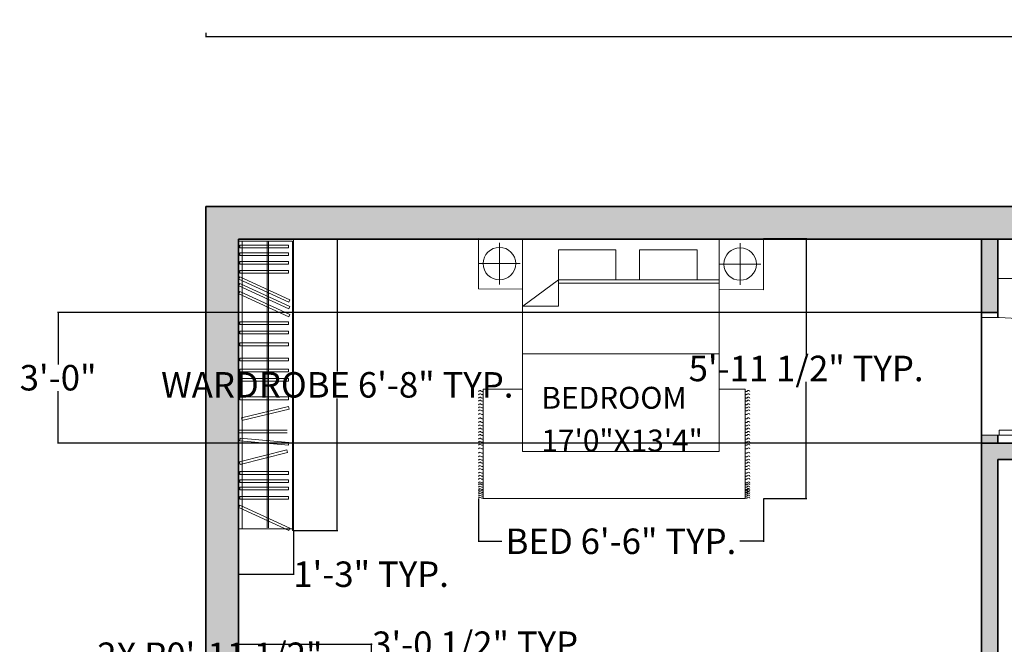
# Model space of a CAD drawing. Units: inches. Extents: x 1319 to 2030, y 219 to 1069.
# Tile 25 of 28: x 1319 to 1589, y 835 to 1007. Entities that reach past the tile are written whole.
import ezdxf

# ---------------------------------------------------------------- set-up
doc = ezdxf.new("R2010")
doc.units = ezdxf.units.IN
doc.header["$MEASUREMENT"] = 0
doc.layers.get('0').update_dxf_attribs({"color": 12})
for name, color, linetype, lineweight in [('A-ANNO-DIMS', 2, 'Continuous', 18), ('A-AREA-IDEN', 250, 'Continuous', 18), ('A-WALL-PATT', 252, 'Continuous', 13), ('C-PROP', 7, 'Continuous', 35), ('closet', 252, 'Continuous', 18), ('doors', 252, 'Continuous', 18), ('furniture', 250, 'Continuous', 18), ('walls', 250, 'Continuous', 35)]:
    doc.layers.add(name, color=color, linetype=linetype, lineweight=lineweight)
doc.styles.get("Standard").update_dxf_attribs({"font": 'arial.ttf'})
doc.dimstyles.get("Standard").update_dxf_attribs({"dimtxt": 7, "dimasz": 0.18, "dimexe": 0.18, "dimexo": 0.0625, "dimgap": 0.09, "dimtad": 0, "dimtih": 1, "dimtoh": 1, "dimzin": 0, "dimdsep": 46, "dimlunit": 3, "dimtxsty": 'Standard', "dimcen": 0.09, "dimadec": 0, "dimazin": 0, "dimtfac": 1, "dimtofl": 0, "dimtmove": 0, "dimatfit": 3, "dimfxl": 1, "dimtolj": 1, "dimtzin": 0, "dimarcsym": 0})

# ---------------------------------------------------------------- blocks, each defined once
blk = doc.blocks.new('*U2')
for p, q in [((0, 0), (0, -6)), ((40, 0), (40, -6))]:
    blk.add_line(p, q)
blk.add_lwpolyline([(0, 0), (0, 40), (1.75, 40), (1.75, 0)], close=True)
blk.add_arc((0, 0), 40, 0, 90)
blk = doc.blocks.new('CARPET')
at = {"layer": 'furniture'}
for p, q in [((-51.53, -98.11), (-51.53, -55.12)), ((-51.53, -55.12), (-41.27, -55.12)), ((36, -55.12), (51.55, -55.12)), ((51.55, -55.12), (51.55, -98.11)), ((51.55, -98.11), (-51.53, -98.11))]:
    blk.add_line(p, q, dxfattribs=at)
for points, knots in [([(-53.37, -55.99), (-53.22, -55.8), (-52.9, -55.41), (-52.34, -55.8), (-51.89, -56.08), (-51.65, -55.91), (-51.53, -55.83)], [0, 0, 0, 0, 0.653278, 1.290138, 1.740457, 2.114451, 2.114451, 2.114451, 2.114451]), ([(-53.37, -57.26), (-53.22, -57.07), (-52.9, -56.67), (-52.34, -57.07), (-51.89, -57.35), (-51.65, -57.17), (-51.53, -57.1)], [0, 0, 0, 0, 0.653278, 1.290138, 1.740457, 2.114451, 2.114451, 2.114451, 2.114451]), ([(53.37, -55.99), (53.22, -55.8), (52.9, -55.41), (52.34, -55.8), (51.89, -56.08), (51.65, -55.91), (51.53, -55.83)], [0, 0, 0, 0, 0.653278, 1.290138, 1.740457, 2.114451, 2.114451, 2.114451, 2.114451]), ([(53.37, -57.26), (53.22, -57.07), (52.9, -56.67), (52.34, -57.07), (51.89, -57.35), (51.65, -57.17), (51.53, -57.1)], [0, 0, 0, 0, 0.653278, 1.290138, 1.740457, 2.114451, 2.114451, 2.114451, 2.114451]), ([(-53.37, -58.59), (-53.22, -58.4), (-52.9, -58.01), (-52.34, -58.4), (-51.89, -58.68), (-51.65, -58.5), (-51.53, -58.43)], [0, 0, 0, 0, 0.653278, 1.290138, 1.740457, 2.114451, 2.114451, 2.114451, 2.114451]), ([(-53.37, -59.78), (-53.22, -59.58), (-52.9, -59.19), (-52.34, -59.58), (-51.89, -59.86), (-51.65, -59.69), (-51.53, -59.61)], [0, 0, 0, 0, 0.653278, 1.290138, 1.740457, 2.114451, 2.114451, 2.114451, 2.114451]), ([(-53.37, -61.22), (-53.22, -61.02), (-52.9, -60.63), (-52.34, -61.02), (-51.89, -61.3), (-51.65, -61.13), (-51.53, -61.05)], [0, 0, 0, 0, 0.653278, 1.290138, 1.740457, 2.114451, 2.114451, 2.114451, 2.114451]), ([(53.37, -58.59), (53.22, -58.4), (52.9, -58.01), (52.34, -58.4), (51.89, -58.68), (51.65, -58.5), (51.53, -58.43)], [0, 0, 0, 0, 0.653278, 1.290138, 1.740457, 2.114451, 2.114451, 2.114451, 2.114451]), ([(53.37, -59.78), (53.22, -59.58), (52.9, -59.19), (52.34, -59.58), (51.89, -59.86), (51.65, -59.69), (51.53, -59.61)], [0, 0, 0, 0, 0.653278, 1.290138, 1.740457, 2.114451, 2.114451, 2.114451, 2.114451]), ([(53.37, -61.22), (53.22, -61.02), (52.9, -60.63), (52.34, -61.02), (51.89, -61.3), (51.65, -61.13), (51.53, -61.05)], [0, 0, 0, 0, 0.653278, 1.290138, 1.740457, 2.114451, 2.114451, 2.114451, 2.114451]), ([(-53.37, -62.44), (-53.22, -62.25), (-52.9, -61.86), (-52.34, -62.25), (-51.89, -62.53), (-51.65, -62.36), (-51.53, -62.28)], [0, 0, 0, 0, 0.653278, 1.290138, 1.740457, 2.114451, 2.114451, 2.114451, 2.114451]), ([(-53.37, -63.63), (-53.22, -63.43), (-52.9, -63.04), (-52.34, -63.43), (-51.89, -63.72), (-51.65, -63.54), (-51.53, -63.46)], [0, 0, 0, 0, 0.653278, 1.290138, 1.740457, 2.114451, 2.114451, 2.114451, 2.114451]), ([(-53.37, -65.07), (-53.22, -64.87), (-52.9, -64.48), (-52.34, -64.87), (-51.89, -65.15), (-51.65, -64.98), (-51.53, -64.9)], [0, 0, 0, 0, 0.653278, 1.290138, 1.740457, 2.114451, 2.114451, 2.114451, 2.114451]), ([(53.37, -62.44), (53.22, -62.25), (52.9, -61.86), (52.34, -62.25), (51.89, -62.53), (51.65, -62.36), (51.53, -62.28)], [0, 0, 0, 0, 0.653278, 1.290138, 1.740457, 2.114451, 2.114451, 2.114451, 2.114451]), ([(53.37, -63.63), (53.22, -63.43), (52.9, -63.04), (52.34, -63.43), (51.89, -63.72), (51.65, -63.54), (51.53, -63.46)], [0, 0, 0, 0, 0.653278, 1.290138, 1.740457, 2.114451, 2.114451, 2.114451, 2.114451]), ([(53.37, -65.07), (53.22, -64.87), (52.9, -64.48), (52.34, -64.87), (51.89, -65.15), (51.65, -64.98), (51.53, -64.9)], [0, 0, 0, 0, 0.653278, 1.290138, 1.740457, 2.114451, 2.114451, 2.114451, 2.114451]), ([(-53.37, -66.76), (-53.22, -66.56), (-52.9, -66.17), (-52.34, -66.56), (-51.89, -66.84), (-51.65, -66.67), (-51.53, -66.59)], [0, 0, 0, 0, 0.653278, 1.290138, 1.740457, 2.114451, 2.114451, 2.114451, 2.114451]), ([(-53.37, -68.2), (-53.22, -68), (-52.9, -67.61), (-52.34, -68), (-51.89, -68.28), (-51.65, -68.11), (-51.53, -68.03)], [0, 0, 0, 0, 0.653278, 1.290138, 1.740457, 2.114451, 2.114451, 2.114451, 2.114451]), ([(-53.37, -69.53), (-53.22, -69.33), (-52.9, -68.94), (-52.34, -69.33), (-51.89, -69.61), (-51.65, -69.44), (-51.53, -69.36)], [0, 0, 0, 0, 0.653278, 1.290138, 1.740457, 2.114451, 2.114451, 2.114451, 2.114451]), ([(53.37, -66.76), (53.22, -66.56), (52.9, -66.17), (52.34, -66.56), (51.89, -66.84), (51.65, -66.67), (51.53, -66.59)], [0, 0, 0, 0, 0.653278, 1.290138, 1.740457, 2.114451, 2.114451, 2.114451, 2.114451]), ([(53.37, -68.2), (53.22, -68), (52.9, -67.61), (52.34, -68), (51.89, -68.28), (51.65, -68.11), (51.53, -68.03)], [0, 0, 0, 0, 0.653278, 1.290138, 1.740457, 2.114451, 2.114451, 2.114451, 2.114451]), ([(53.37, -69.53), (53.22, -69.33), (52.9, -68.94), (52.34, -69.33), (51.89, -69.61), (51.65, -69.44), (51.53, -69.36)], [0, 0, 0, 0, 0.653278, 1.290138, 1.740457, 2.114451, 2.114451, 2.114451, 2.114451]), ([(-53.37, -70.79), (-53.22, -70.6), (-52.9, -70.21), (-52.34, -70.6), (-51.89, -70.88), (-51.65, -70.7), (-51.53, -70.63)], [0, 0, 0, 0, 0.653278, 1.290138, 1.740457, 2.114451, 2.114451, 2.114451, 2.114451]), ([(-53.37, -72.12), (-53.22, -71.93), (-52.9, -71.54), (-52.34, -71.93), (-51.89, -72.21), (-51.65, -72.04), (-51.53, -71.96)], [0, 0, 0, 0, 0.653278, 1.290138, 1.740457, 2.114451, 2.114451, 2.114451, 2.114451]), ([(-53.37, -73.31), (-53.22, -73.11), (-52.9, -72.72), (-52.34, -73.11), (-51.89, -73.4), (-51.65, -73.22), (-51.53, -73.14)], [0, 0, 0, 0, 0.653278, 1.290138, 1.740457, 2.114451, 2.114451, 2.114451, 2.114451]), ([(53.37, -70.79), (53.22, -70.6), (52.9, -70.21), (52.34, -70.6), (51.89, -70.88), (51.65, -70.7), (51.53, -70.63)], [0, 0, 0, 0, 0.653278, 1.290138, 1.740457, 2.114451, 2.114451, 2.114451, 2.114451]), ([(53.37, -72.12), (53.22, -71.93), (52.9, -71.54), (52.34, -71.93), (51.89, -72.21), (51.65, -72.04), (51.53, -71.96)], [0, 0, 0, 0, 0.653278, 1.290138, 1.740457, 2.114451, 2.114451, 2.114451, 2.114451]), ([(53.37, -73.31), (53.22, -73.11), (52.9, -72.72), (52.34, -73.11), (51.89, -73.4), (51.65, -73.22), (51.53, -73.14)], [0, 0, 0, 0, 0.653278, 1.290138, 1.740457, 2.114451, 2.114451, 2.114451, 2.114451]), ([(-53.37, -74.75), (-53.22, -74.55), (-52.9, -74.16), (-52.34, -74.55), (-51.89, -74.83), (-51.65, -74.66), (-51.53, -74.58)], [0, 0, 0, 0, 0.653278, 1.290138, 1.740457, 2.114451, 2.114451, 2.114451, 2.114451]), ([(-53.37, -75.98), (-53.22, -75.78), (-52.9, -75.39), (-52.34, -75.78), (-51.89, -76.06), (-51.65, -75.89), (-51.53, -75.81)], [0, 0, 0, 0, 0.653278, 1.290138, 1.740457, 2.114451, 2.114451, 2.114451, 2.114451]), ([(-53.37, -77.16), (-53.22, -76.96), (-52.9, -76.57), (-52.34, -76.96), (-51.89, -77.25), (-51.65, -77.07), (-51.53, -76.99)], [0, 0, 0, 0, 0.653278, 1.290138, 1.740457, 2.114451, 2.114451, 2.114451, 2.114451]), ([(53.37, -74.75), (53.22, -74.55), (52.9, -74.16), (52.34, -74.55), (51.89, -74.83), (51.65, -74.66), (51.53, -74.58)], [0, 0, 0, 0, 0.653278, 1.290138, 1.740457, 2.114451, 2.114451, 2.114451, 2.114451]), ([(53.37, -75.98), (53.22, -75.78), (52.9, -75.39), (52.34, -75.78), (51.89, -76.06), (51.65, -75.89), (51.53, -75.81)], [0, 0, 0, 0, 0.653278, 1.290138, 1.740457, 2.114451, 2.114451, 2.114451, 2.114451]), ([(53.37, -77.16), (53.22, -76.96), (52.9, -76.57), (52.34, -76.96), (51.89, -77.25), (51.65, -77.07), (51.53, -76.99)], [0, 0, 0, 0, 0.653278, 1.290138, 1.740457, 2.114451, 2.114451, 2.114451, 2.114451]), ([(-53.37, -78.6), (-53.22, -78.4), (-52.9, -78.01), (-52.34, -78.4), (-51.89, -78.68), (-51.65, -78.51), (-51.53, -78.43)], [0, 0, 0, 0, 0.653278, 1.290138, 1.740457, 2.114451, 2.114451, 2.114451, 2.114451]), ([(-53.37, -80.29), (-53.22, -80.09), (-52.9, -79.7), (-52.34, -80.09), (-51.89, -80.37), (-51.65, -80.2), (-51.53, -80.12)], [0, 0, 0, 0, 0.653278, 1.290138, 1.740457, 2.114451, 2.114451, 2.114451, 2.114451]), ([(-53.37, -81.73), (-53.22, -81.53), (-52.9, -81.14), (-52.34, -81.53), (-51.89, -81.81), (-51.65, -81.64), (-51.53, -81.56)], [0, 0, 0, 0, 0.653278, 1.290138, 1.740457, 2.114451, 2.114451, 2.114451, 2.114451]), ([(53.37, -78.6), (53.22, -78.4), (52.9, -78.01), (52.34, -78.4), (51.89, -78.68), (51.65, -78.51), (51.53, -78.43)], [0, 0, 0, 0, 0.653278, 1.290138, 1.740457, 2.114451, 2.114451, 2.114451, 2.114451]), ([(53.37, -80.29), (53.22, -80.09), (52.9, -79.7), (52.34, -80.09), (51.89, -80.37), (51.65, -80.2), (51.53, -80.12)], [0, 0, 0, 0, 0.653278, 1.290138, 1.740457, 2.114451, 2.114451, 2.114451, 2.114451]), ([(53.37, -81.73), (53.22, -81.53), (52.9, -81.14), (52.34, -81.53), (51.89, -81.81), (51.65, -81.64), (51.53, -81.56)], [0, 0, 0, 0, 0.653278, 1.290138, 1.740457, 2.114451, 2.114451, 2.114451, 2.114451]), ([(-53.37, -83.06), (-53.22, -82.86), (-52.9, -82.47), (-52.34, -82.86), (-51.89, -83.14), (-51.65, -82.97), (-51.53, -82.89)], [0, 0, 0, 0, 0.653278, 1.290138, 1.740457, 2.114451, 2.114451, 2.114451, 2.114451]), ([(-53.37, -84.18), (-53.22, -83.99), (-52.9, -83.6), (-52.34, -83.99), (-51.89, -84.27), (-51.65, -84.09), (-51.53, -84.02)], [0, 0, 0, 0, 0.653278, 1.290138, 1.740457, 2.114451, 2.114451, 2.114451, 2.114451]), ([(-53.37, -85.51), (-53.22, -85.32), (-52.9, -84.93), (-52.34, -85.32), (-51.89, -85.6), (-51.65, -85.42), (-51.53, -85.35)], [0, 0, 0, 0, 0.653278, 1.290138, 1.740457, 2.114451, 2.114451, 2.114451, 2.114451]), ([(53.37, -83.06), (53.22, -82.86), (52.9, -82.47), (52.34, -82.86), (51.89, -83.14), (51.65, -82.97), (51.53, -82.89)], [0, 0, 0, 0, 0.653278, 1.290138, 1.740457, 2.114451, 2.114451, 2.114451, 2.114451]), ([(53.37, -84.18), (53.22, -83.99), (52.9, -83.6), (52.34, -83.99), (51.89, -84.27), (51.65, -84.09), (51.53, -84.02)], [0, 0, 0, 0, 0.653278, 1.290138, 1.740457, 2.114451, 2.114451, 2.114451, 2.114451]), ([(53.37, -85.51), (53.22, -85.32), (52.9, -84.93), (52.34, -85.32), (51.89, -85.6), (51.65, -85.42), (51.53, -85.35)], [0, 0, 0, 0, 0.653278, 1.290138, 1.740457, 2.114451, 2.114451, 2.114451, 2.114451]), ([(-53.37, -86.7), (-53.22, -86.5), (-52.9, -86.11), (-52.34, -86.5), (-51.89, -86.78), (-51.65, -86.61), (-51.53, -86.53)], [0, 0, 0, 0, 0.653278, 1.290138, 1.740457, 2.114451, 2.114451, 2.114451, 2.114451]), ([(-53.37, -88.14), (-53.22, -87.94), (-52.9, -87.55), (-52.34, -87.94), (-51.89, -88.22), (-51.65, -88.05), (-51.53, -87.97)], [0, 0, 0, 0, 0.653278, 1.290138, 1.740457, 2.114451, 2.114451, 2.114451, 2.114451]), ([(-53.37, -89.36), (-53.22, -89.17), (-52.9, -88.78), (-52.34, -89.17), (-51.89, -89.45), (-51.65, -89.28), (-51.53, -89.2)], [0, 0, 0, 0, 0.653278, 1.290138, 1.740457, 2.114451, 2.114451, 2.114451, 2.114451]), ([(53.37, -86.7), (53.22, -86.5), (52.9, -86.11), (52.34, -86.5), (51.89, -86.78), (51.65, -86.61), (51.53, -86.53)], [0, 0, 0, 0, 0.653278, 1.290138, 1.740457, 2.114451, 2.114451, 2.114451, 2.114451]), ([(53.37, -88.14), (53.22, -87.94), (52.9, -87.55), (52.34, -87.94), (51.89, -88.22), (51.65, -88.05), (51.53, -87.97)], [0, 0, 0, 0, 0.653278, 1.290138, 1.740457, 2.114451, 2.114451, 2.114451, 2.114451]), ([(53.37, -89.36), (53.22, -89.17), (52.9, -88.78), (52.34, -89.17), (51.89, -89.45), (51.65, -89.28), (51.53, -89.2)], [0, 0, 0, 0, 0.653278, 1.290138, 1.740457, 2.114451, 2.114451, 2.114451, 2.114451]), ([(-53.37, -90.55), (-53.22, -90.35), (-52.9, -89.96), (-52.34, -90.35), (-51.89, -90.64), (-51.65, -90.46), (-51.53, -90.38)], [0, 0, 0, 0, 0.653278, 1.290138, 1.740457, 2.114451, 2.114451, 2.114451, 2.114451]), ([(-53.37, -91.99), (-53.22, -91.79), (-52.9, -91.4), (-52.34, -91.79), (-51.89, -92.07), (-51.65, -91.9), (-51.53, -91.82)], [0, 0, 0, 0, 0.653278, 1.290138, 1.740457, 2.114451, 2.114451, 2.114451, 2.114451]), ([(-53.37, -92.69), (-53.22, -92.48), (-52.9, -92.08), (-52.35, -92.49), (-51.89, -92.77), (-51.65, -92.6), (-51.53, -92.52)], [0, 0, 0, 0, 0.663904, 1.307406, 1.757725, 2.131719, 2.131719, 2.131719, 2.131719]), ([(53.37, -90.55), (53.22, -90.35), (52.9, -89.96), (52.34, -90.35), (51.9, -90.63), (51.66, -90.47), (51.55, -90.4)], [0, 0, 0, 0, 0.653278, 1.290138, 1.740457, 2.0926, 2.0926, 2.0926, 2.0926]), ([(53.37, -91.99), (53.22, -91.79), (52.9, -91.4), (52.34, -91.79), (51.9, -92.07), (51.66, -91.91), (51.55, -91.83)], [0, 0, 0, 0, 0.653278, 1.290138, 1.740457, 2.0926, 2.0926, 2.0926, 2.0926]), ([(53.37, -92.69), (53.22, -92.49), (52.9, -92.09), (52.34, -92.49), (51.9, -92.77), (51.66, -92.61), (51.55, -92.53)], [0, 0, 0, 0, 0.656792, 1.295826, 1.746145, 2.098292, 2.098292, 2.098292, 2.098292]), ([(-53.37, -93.61), (-53.22, -93.42), (-52.9, -93.03), (-52.34, -93.42), (-51.89, -93.7), (-51.65, -93.52), (-51.53, -93.45)], [0, 0, 0, 0, 0.653278, 1.290138, 1.740457, 2.114451, 2.114451, 2.114451, 2.114451]), ([(-53.37, -94.55), (-53.22, -94.35), (-52.9, -93.96), (-52.34, -94.35), (-51.89, -94.63), (-51.65, -94.46), (-51.53, -94.38)], [0, 0, 0, 0, 0.653278, 1.290138, 1.740457, 2.114451, 2.114451, 2.114451, 2.114451]), ([(-53.37, -95.05), (-53.22, -94.85), (-52.9, -94.46), (-52.34, -94.85), (-51.89, -95.14), (-51.65, -94.96), (-51.53, -94.88)], [0, 0, 0, 0, 0.653278, 1.290138, 1.740457, 2.114451, 2.114451, 2.114451, 2.114451]), ([(-53.37, -95.73), (-53.22, -95.54), (-52.9, -95.15), (-52.34, -95.54), (-51.89, -95.82), (-51.65, -95.65), (-51.53, -95.57)], [0, 0, 0, 0, 0.653278, 1.290138, 1.740457, 2.114451, 2.114451, 2.114451, 2.114451]), ([(-53.37, -96.38), (-53.22, -96.18), (-52.9, -95.79), (-52.34, -96.18), (-51.89, -96.47), (-51.65, -96.29), (-51.53, -96.21)], [0, 0, 0, 0, 0.653278, 1.290138, 1.740457, 2.114451, 2.114451, 2.114451, 2.114451]), ([(-53.37, -97.17), (-53.22, -96.98), (-52.9, -96.59), (-52.34, -96.98), (-51.89, -97.26), (-51.65, -97.08), (-51.53, -97.01)], [0, 0, 0, 0, 0.653278, 1.290138, 1.740457, 2.114451, 2.114451, 2.114451, 2.114451]), ([(53.37, -95.78), (53.22, -95.58), (52.9, -95.19), (52.34, -95.58), (51.89, -95.86), (51.65, -95.69), (51.53, -95.61)], [0, 0, 0, 0, 0.653278, 1.290138, 1.740457, 2.114451, 2.114451, 2.114451, 2.114451]), ([(53.37, -96.43), (53.22, -96.23), (52.9, -95.84), (52.34, -96.23), (51.89, -96.51), (51.65, -96.34), (51.53, -96.26)], [0, 0, 0, 0, 0.653278, 1.290138, 1.740457, 2.114451, 2.114451, 2.114451, 2.114451]), ([(53.37, -93.66), (53.22, -93.46), (52.9, -93.07), (52.34, -93.46), (51.9, -93.74), (51.66, -93.58), (51.55, -93.5)], [0, 0, 0, 0, 0.653278, 1.290138, 1.740457, 2.0926, 2.0926, 2.0926, 2.0926]), ([(53.37, -94.59), (53.22, -94.4), (52.9, -94.01), (52.34, -94.4), (51.9, -94.68), (51.66, -94.51), (51.55, -94.44)], [0, 0, 0, 0, 0.653278, 1.290138, 1.740457, 2.0926, 2.0926, 2.0926, 2.0926]), ([(53.37, -95.1), (53.22, -94.9), (52.9, -94.51), (52.34, -94.9), (51.9, -95.18), (51.66, -95.02), (51.55, -94.94)], [0, 0, 0, 0, 0.653278, 1.290138, 1.740457, 2.0926, 2.0926, 2.0926, 2.0926]), ([(-53.37, -97.99), (-53.22, -97.79), (-52.9, -97.4), (-52.34, -97.79), (-51.89, -98.08), (-51.65, -97.9), (-51.53, -97.82)], [0, 0, 0, 0, 0.653278, 1.290138, 1.740457, 2.114451, 2.114451, 2.114451, 2.114451]), ([(53.37, -97.22), (53.22, -97.02), (52.9, -96.63), (52.34, -97.02), (51.89, -97.3), (51.65, -97.13), (51.53, -97.05)], [0, 0, 0, 0, 0.653278, 1.290138, 1.740457, 2.114451, 2.114451, 2.114451, 2.114451]), ([(53.37, -97.99), (53.22, -97.79), (52.9, -97.4), (52.34, -97.79), (51.89, -98.08), (51.65, -97.9), (51.53, -97.82)], [0, 0, 0, 0, 0.653278, 1.290138, 1.740457, 2.114451, 2.114451, 2.114451, 2.114451])]:
    blk.add_open_spline(points, degree=3, knots=knots, dxfattribs=at)
blk = doc.blocks.new('A$C58D270C6')
at = {"layer": 'furniture'}
for p, q in [((9.09, 124.13), (9.09, 108.87)), ((1.46, 116.5), (16.73, 116.5)), ((14.97, 94.84), (24.62, 107.92)), ((24.62, 94.93), (24.62, 107.92)), ((42.08, 108), (42.08, 36)), ((14.97, 94.93), (24.62, 94.93)), ((14.97, 94.84), (14.97, 36)), ((16.22, 94.93), (16.22, 36)), ((9.25, 36), (9.25, 20.74)), ((1.62, 28.37), (16.88, 28.37))]:
    blk.add_line(p, q, dxfattribs=at)
for points in [[(18.5, 108), (18.34, 124.13), (-0.16, 124.13), (0, 108)], [(0, 108), (77.91, 108), (77.91, 36), (0, 36)], [(4.09, 94.93), (14.97, 94.93), (14.97, 73.83), (4.09, 73.83)], [(4.09, 65.23), (14.97, 65.23), (14.97, 44.13), (4.09, 44.13)], [(18.65, 19.87), (18.5, 36), (0, 36), (0.16, 19.87)]]:
    blk.add_lwpolyline(points, close=True, dxfattribs=at)
for centre in [(9.09, 116.5), (9.25, 28.37)]:
    blk.add_circle(centre, 5.95, dxfattribs=at)
at = {"layer": 'furniture', "xscale": 0.9312884925094044, "yscale": 0.9312884925094044, "zscale": 0.9312884925094044, "rotation": 90}
blk.add_blockref('CARPET', (3.79, 74.47), dxfattribs=at)
blk = doc.blocks.new('*D28')
at = {"layer": 'A-ANNO-DIMS', "color": 0, "lineweight": -2, "transparency": 16777216}
for p, q in [((1369.84, 1002.94), (1369.84, 1001.77)), ((1370.02, 1001.95), (1663.81, 1001.95)), ((1969.66, 1001.95), (1675.87, 1001.95)), ((1969.84, 1002.94), (1969.84, 1001.77))]:
    blk.add_line(p, q, dxfattribs=at)
at = {"layer": 'A-ANNO-DIMS', "color": 0, "transparency": 16777216}
for points in [[(1370.02, 1001.98), (1370.02, 1001.92), (1369.84, 1001.95)], [(1969.66, 1001.98), (1969.66, 1001.92), (1969.84, 1001.95)]]:
    blk.add_solid(points, dxfattribs=at)
at = {"layer": 'Defpoints', "color": 0, "transparency": 16777216}
for p in [(1369.84, 1003), (1969.84, 1003), (1969.84, 1001.95)]:
    blk.add_point(p, dxfattribs=at)
at = {"layer": 'A-ANNO-DIMS', "color": 0, "transparency": 16777216, "insert": (1669.84, 1001.95), "char_height": 7, "attachment_point": 5}
blk.add_mtext("\\A1;50'", dxfattribs=at)
blk = doc.blocks.new('closet')
at = {"layer": 'closet'}
for p, q in [((-0.71, -5.58), (5.59, 8.19)), ((5.59, 8.19), (6.27, 7.88)), ((26.09, 8.25), (26.09, -5.1)), ((26.84, 8.25), (26.84, -5.1)), ((57.99, -5.58), (64.3, 8.19)), ((60.19, -5.58), (66.49, 8.19)), ((62, -5.58), (68.3, 8.19)), ((-0.23, 7.39), (-0.23, -6.57)), ((6.27, 7.88), (-0.04, -5.89)), ((7.92, 7.84), (8.68, 7.84)), ((7.92, 7.84), (7.92, -5.51)), ((8.68, 7.84), (8.68, -5.51)), ((10.44, 7.84), (11.2, 7.84)), ((10.44, 7.84), (10.44, -5.51)), ((11.2, 7.84), (11.2, -5.51)), ((12.45, 7.84), (13.21, 7.84)), ((12.45, 7.84), (12.45, -5.51)), ((13.21, 7.84), (13.21, -5.51)), ((14.71, 7.84), (15.47, 7.84)), ((14.71, 7.84), (14.71, -5.51)), ((15.47, 7.84), (15.47, -5.51)), ((17.44, 7.75), (18.17, 7.93)), ((17.44, 7.75), (20.73, -5.2)), ((18.17, 7.93), (21.46, -5.01)), ((23.92, 7.84), (22.75, -5.46)), ((24.67, 7.78), (23.51, -5.53)), ((23.92, 7.84), (24.67, 7.78)), ((29.49, 7.29), (32.64, -5.69)), ((30.22, 7.46), (33.37, -5.51)), ((35.23, 7.84), (35.23, -5.51)), ((35.99, 7.84), (35.99, -5.51)), ((40.33, 7.84), (40.33, -5.51)), ((41.08, 7.84), (41.08, -5.51)), ((42.85, 7.84), (42.85, -5.51)), ((43.61, 7.84), (43.61, -5.51)), ((45.9, 7.84), (45.9, -5.51)), ((46.65, 7.84), (46.65, -5.51)), ((50.07, 7.84), (50.07, -5.51)), ((50.82, 7.84), (50.82, -5.51)), ((53.32, 7.84), (53.32, -5.51)), ((54.08, 7.84), (54.08, -5.51)), ((55.9, 7.84), (55.9, -5.51)), ((56.65, 7.84), (56.65, -5.51)), ((64.97, 7.88), (58.67, -5.89)), ((67.17, 7.88), (60.87, -5.89)), ((68.98, 7.88), (62.67, -5.89)), ((69.96, 7.84), (69.96, -5.51)), ((70.72, 7.84), (70.72, -5.51)), ((72.43, 7.84), (72.43, -5.51)), ((73.19, 7.84), (73.19, -5.51)), ((74.82, 7.84), (74.82, -5.51)), ((75.57, 7.84), (75.57, -5.51)), ((76.94, 7.84), (76.94, -5.51)), ((77.69, 7.84), (77.69, -5.51)), ((56.23, 0.33), (0, 0.33)), ((56.2, 0), (0, 0)), ((56.2, 0), (78.76, 0)), ((56.23, 0.33), (78.76, 0.33)), ((21.46, -5.01), (20.73, -5.2)), ((-0.04, -5.89), (-0.71, -5.58)), ((23.51, -5.53), (22.75, -5.46)), ((33.37, -5.51), (32.64, -5.69)), ((35.99, -5.51), (35.23, -5.51)), ((41.08, -5.51), (40.33, -5.51)), ((43.61, -5.51), (42.85, -5.51)), ((46.65, -5.51), (45.9, -5.51)), ((50.82, -5.51), (50.07, -5.51)), ((54.08, -5.51), (53.32, -5.51)), ((56.65, -5.51), (55.9, -5.51)), ((58.67, -5.89), (57.99, -5.58)), ((60.87, -5.89), (60.19, -5.58)), ((62.67, -5.89), (62, -5.58)), ((70.72, -5.51), (69.96, -5.51)), ((73.19, -5.51), (72.43, -5.51)), ((75.57, -5.51), (74.82, -5.51)), ((77.69, -5.51), (76.94, -5.51))]:
    blk.add_line(p, q, dxfattribs=at)
blk = doc.blocks.new('rotated closet')
at = {"layer": 'closet'}
for p, q in [((26.32, 0.86), (27.07, 0.86)), ((29.72, -0.11), (30.45, 0.07)), ((35.46, 0.45), (36.22, 0.45)), ((40.56, 0.45), (41.31, 0.45)), ((43.08, 0.45), (43.84, 0.45)), ((46.13, 0.45), (46.88, 0.45)), ((50.3, 0.45), (51.05, 0.45)), ((53.56, 0.45), (54.31, 0.45)), ((56.13, 0.45), (56.88, 0.45)), ((64.53, 0.8), (65.2, 0.49)), ((66.72, 0.8), (67.4, 0.49)), ((68.53, 0.8), (69.21, 0.49)), ((70.19, 0.45), (70.95, 0.45)), ((72.66, 0.45), (73.42, 0.45)), ((75.05, 0.45), (75.81, 0.45)), ((77.17, 0.45), (77.92, 0.45)), ((78.99, 0), (78.99, -13.96)), ((8.91, -12.91), (8.15, -12.91)), ((11.43, -12.91), (10.67, -12.91)), ((13.44, -12.91), (12.68, -12.91)), ((15.7, -12.91), (14.94, -12.91)), ((-0.46, -14.27), (79.54, -14.27)), ((0, -13.96), (78.99, -13.96))]:
    blk.add_line(p, q, dxfattribs=at)
blk.add_blockref('closet', (0.23, -7.39), dxfattribs=at)
blk = doc.blocks.new('WARDROBE-80')
for p, q in [((14.82, 79.47), (0.01, 79.47)), ((0.01, 0.48), (0.01, 79.47)), ((1.04, 79.35), (1.04, 0.36)), ((14.82, 0.48), (14.82, 79.47)), ((15.13, 0.02), (15.13, 80.02)), ((15.13, 0.02), (15.13, 80.02)), ((15.13, 0.02), (15.13, 80.02)), ((15.13, 77.37), (15.13, 79.47)), ((15.13, 77.37), (15.13, 79.47)), ((14.82, 0.48), (14.82, 77.83)), ((0.01, 0.48), (14.82, 0.48)), ((14.82, 0.02), (14.82, 0.48)), ((15.13, 0.02), (14.82, 0.02))]:
    blk.add_line(p, q)
at = {"rotation": 89.99999999920078}
blk.add_blockref('rotated closet', (0.86, 0.48), dxfattribs=at)
blk = doc.blocks.new('*D42')
at = {"layer": 'A-ANNO-DIMS', "color": 0, "lineweight": -2, "transparency": 16777216}
for p, q in [((1444.72, 874.91), (1444.72, 863.06)), ((1522.95, 874.91), (1522.95, 863.06)), ((1444.9, 863.24), (1451.16, 863.24)), ((1522.77, 863.24), (1516.52, 863.24))]:
    blk.add_line(p, q, dxfattribs=at)
at = {"layer": 'A-ANNO-DIMS', "color": 0, "transparency": 16777216}
for points in [[(1444.9, 863.27), (1444.9, 863.21), (1444.72, 863.24)], [(1522.77, 863.27), (1522.77, 863.21), (1522.95, 863.24)]]:
    blk.add_solid(points, dxfattribs=at)
at = {"layer": 'Defpoints', "color": 0, "transparency": 16777216}
for p in [(1444.72, 874.97), (1522.95, 874.97), (1444.72, 863.24)]:
    blk.add_point(p, dxfattribs=at)
at = {"layer": 'A-ANNO-DIMS', "color": 0, "transparency": 16777216, "insert": (1483.84, 863.24), "char_height": 7, "attachment_point": 5}
blk.add_mtext('\\A1;BED 6\'-6" TYP.', dxfattribs=at)
blk = doc.blocks.new('*D43')
at = {"layer": 'A-ANNO-DIMS', "color": 0, "lineweight": -2, "transparency": 16777216}
for p, q in [((1523.02, 946.46), (1534.87, 946.46)), ((1534.69, 946.28), (1534.69, 914.43)), ((1534.69, 875.15), (1534.69, 907.01)), ((1523.02, 874.97), (1534.87, 874.97))]:
    blk.add_line(p, q, dxfattribs=at)
at = {"layer": 'A-ANNO-DIMS', "color": 0, "transparency": 16777216}
for points in [[(1534.66, 946.28), (1534.72, 946.28), (1534.69, 946.46)], [(1534.66, 875.15), (1534.72, 875.15), (1534.69, 874.97)]]:
    blk.add_solid(points, dxfattribs=at)
at = {"layer": 'Defpoints', "color": 0, "transparency": 16777216}
for p in [(1522.95, 946.46), (1522.95, 874.97), (1534.69, 874.97)]:
    blk.add_point(p, dxfattribs=at)
at = {"layer": 'A-ANNO-DIMS', "color": 0, "transparency": 16777216, "insert": (1534.69, 910.72), "char_height": 7, "attachment_point": 5}
blk.add_mtext('\\A1;5\'-11 1/2" TYP.', dxfattribs=at)
blk = doc.blocks.new('*D47')
at = {"layer": 'A-ANNO-DIMS', "color": 0, "lineweight": -2, "transparency": 16777216}
for p, q in [((1378.84, 828.66), (1378.84, 835.14)), ((1379.02, 834.96), (1415.19, 834.96)), ((1415.37, 828.66), (1415.37, 835.14)), ((1415.37, 834.96), (1415.55, 834.96))]:
    blk.add_line(p, q, dxfattribs=at)
at = {"layer": 'A-ANNO-DIMS', "color": 0, "transparency": 16777216}
for points in [[(1379.02, 834.99), (1379.02, 834.93), (1378.84, 834.96)], [(1415.19, 834.99), (1415.19, 834.93), (1415.37, 834.96)]]:
    blk.add_solid(points, dxfattribs=at)
at = {"layer": 'Defpoints', "color": 0, "transparency": 16777216}
for p in [(1415.37, 834.96), (1378.84, 828.6), (1415.37, 828.6)]:
    blk.add_point(p, dxfattribs=at)
at = {"layer": 'A-ANNO-DIMS', "color": 0, "transparency": 16777216, "insert": (1445.13, 834.96), "char_height": 7, "attachment_point": 5}
blk.add_mtext('\\A1;3\'-0 1/2" TYP.', dxfattribs=at)
blk = doc.blocks.new('*D48')
at = {"layer": 'A-ANNO-DIMS', "color": 0, "lineweight": -2, "transparency": 16777216}
for p, q in [((1394.02, 946.23), (1406.14, 946.23)), ((1405.96, 946.05), (1405.96, 909.93)), ((1405.96, 866.38), (1405.96, 902.5)), ((1394.02, 866.2), (1406.14, 866.2))]:
    blk.add_line(p, q, dxfattribs=at)
at = {"layer": 'A-ANNO-DIMS', "color": 0, "transparency": 16777216}
for points in [[(1405.93, 946.05), (1405.99, 946.05), (1405.96, 946.23)], [(1405.93, 866.38), (1405.99, 866.38), (1405.96, 866.2)]]:
    blk.add_solid(points, dxfattribs=at)
at = {"layer": 'Defpoints', "color": 0, "transparency": 16777216}
for p in [(1393.96, 946.23), (1405.96, 946.23), (1393.96, 866.2)]:
    blk.add_point(p, dxfattribs=at)
at = {"layer": 'A-ANNO-DIMS', "color": 0, "transparency": 16777216, "insert": (1405.96, 906.22), "char_height": 7, "attachment_point": 5}
blk.add_mtext('\\A1;WARDROBE 6\'-8" TYP.', dxfattribs=at)
blk = doc.blocks.new('*D49')
at = {"layer": 'A-ANNO-DIMS', "color": 0, "lineweight": -2, "transparency": 16777216}
for p, q in [((1378.82, 866.14), (1378.82, 854.02)), ((1393.96, 866.14), (1393.96, 854.02)), ((1379, 854.2), (1393.78, 854.2)), ((1393.96, 854.2), (1394.14, 854.2))]:
    blk.add_line(p, q, dxfattribs=at)
at = {"layer": 'A-ANNO-DIMS', "color": 0, "transparency": 16777216}
for points in [[(1379, 854.23), (1379, 854.17), (1378.82, 854.2)], [(1393.78, 854.23), (1393.78, 854.17), (1393.96, 854.2)]]:
    blk.add_solid(points, dxfattribs=at)
at = {"layer": 'Defpoints', "color": 0, "transparency": 16777216}
for p in [(1378.82, 866.2), (1393.96, 866.2), (1393.96, 854.2)]:
    blk.add_point(p, dxfattribs=at)
at = {"layer": 'A-ANNO-DIMS', "color": 0, "transparency": 16777216, "insert": (1415.23, 854.2), "char_height": 7, "attachment_point": 5}
blk.add_mtext('\\A1;1\'-3" TYP.', dxfattribs=at)
blk = doc.blocks.new('*D69')
at = {"layer": 'A-ANNO-DIMS', "color": 0, "lineweight": -2, "transparency": 16777216}
for p, q in [((1582.78, 926.14), (1329.11, 926.14)), ((1329.29, 925.96), (1329.29, 911.85)), ((1329.29, 890.41), (1329.29, 904.52)), ((1582.78, 890.23), (1329.11, 890.23))]:
    blk.add_line(p, q, dxfattribs=at)
at = {"layer": 'A-ANNO-DIMS', "color": 0, "transparency": 16777216}
for points in [[(1329.26, 925.96), (1329.32, 925.96), (1329.29, 926.14)], [(1329.26, 890.41), (1329.32, 890.41), (1329.29, 890.23)]]:
    blk.add_solid(points, dxfattribs=at)
at = {"layer": 'Defpoints', "color": 0, "transparency": 16777216}
for p in [(1329.29, 926.14), (1582.84, 926.14), (1582.84, 890.23)]:
    blk.add_point(p, dxfattribs=at)
at = {"layer": 'A-ANNO-DIMS', "color": 0, "transparency": 16777216, "insert": (1329.29, 908.18), "char_height": 7, "attachment_point": 5}
blk.add_mtext('\\A1;3\'-0"', dxfattribs=at)
blk = doc.blocks.new('*D72')
at = {"layer": 'A-ANNO-DIMS', "color": 0, "lineweight": -2, "transparency": 16777216}
for p, q in [((1402.16, 831.93), (1402.34, 831.93)), ((1402.34, 831.93), (1402.34, 825.19)), ((1402.25, 813.46), (1402.43, 813.46)), ((1402.34, 813.37), (1402.34, 813.55))]:
    blk.add_line(p, q, dxfattribs=at)
at = {"layer": 'A-ANNO-DIMS', "color": 0, "transparency": 16777216}
blk.add_solid([(1402.37, 825.19), (1402.31, 825.19), (1402.34, 825.01)], dxfattribs=at)
at = {"layer": 'Defpoints', "color": 0, "transparency": 16777216}
for p in [(1402.34, 825.01), (1402.34, 813.46)]:
    blk.add_point(p, dxfattribs=at)
at = {"layer": 'A-ANNO-DIMS', "color": 0, "transparency": 16777216, "insert": (1370.96, 831.93), "char_height": 7, "attachment_point": 5}
blk.add_mtext('\\A1;2X R0\'-11 1/2"', dxfattribs=at)

msp = doc.modelspace()

# ---------------------------------------------------------------- hatches: boundary and pattern name
at = {"layer": 'A-WALL-PATT'}
h = msp.add_hatch(color=256, dxfattribs=at)
h.dxf.hatch_style = 1
h.paths.add_polyline_path([(1378.843, 946.227), (1960.843, 946.227), (1960.843, 860.616), (1922.194, 860.616), (1922.194, 851.616), (1960.843, 851.616), (1960.843, 304.227), (1578.343, 304.227), (1578.343, 295.227), (1969.843, 295.227), (1969.843, 955.227), (1369.843, 955.227), (1369.843, 295.227), (1378.843, 295.227)])
h = msp.add_hatch(color=256, dxfattribs=at)
h.dxf.hatch_style = 1
h.paths.add_polyline_path([(1856.292, 860.616), (1812.343, 860.616), (1812.343, 851.616), (1812.343, 700.993), (1816.843, 700.993), (1816.843, 851.616), (1856.292, 851.616)])
h.paths.add_polyline_path([(1960.843, 663.616), (1812.343, 663.616), (1782.783, 663.616), (1782.783, 659.116), (1812.343, 659.116), (1960.843, 659.116)])
h.paths.add_polyline_path([(1857.424, 659.116), (1852.924, 659.116), (1852.924, 616.807), (1857.424, 616.807)])
h.paths.add_polyline_path([(1735.843, 661.727), (1731.843, 661.727), (1636.133, 661.727), (1636.133, 657.227), (1731.343, 657.227), (1731.343, 481.227), (1618.616, 481.227), (1618.616, 472.227), (1639.343, 472.227), (1639.343, 384.227), (1627.044, 384.227), (1627.044, 375.227), (1648.343, 375.227), (1648.343, 384.227), (1648.343, 472.227), (1750.706, 472.227), (1750.706, 481.227), (1735.843, 481.227), (1735.843, 657.727)])
h.paths.add_polyline_path([(1587.343, 481.227), (1578.343, 481.227), (1578.343, 375.227), (1597.622, 375.227), (1597.622, 384.227), (1587.343, 384.227)])
h.paths.add_polyline_path([(1769.593, 384.227), (1693.482, 384.227), (1693.482, 375.227), (1769.593, 375.227)])
h.paths.add_polyline_path([(1775.828, 481.227), (1765.831, 481.227), (1765.831, 472.227), (1775.828, 472.227)])
h.paths.add_polyline_path([(1824.625, 481.227), (1820.343, 481.227), (1820.343, 476.727), (1824.625, 476.727), (1824.625, 477.545)], flags=0)
h.paths.add_polyline_path([(1896.843, 481.227), (1852.26, 481.227), (1852.26, 476.727), (1892.343, 476.727), (1892.343, 384.227), (1881.742, 384.227), (1881.742, 375.227), (1913.435, 375.227), (1913.435, 384.227), (1896.843, 384.227)])
h.paths.add_polyline_path([(1960.843, 481.227), (1931.341, 481.227), (1931.341, 476.727), (1960.843, 476.727)])
h.paths.add_polyline_path([(1736.343, 918.227), (1731.843, 918.227), (1731.843, 890.227), (1582.843, 890.227), (1582.843, 781.727), (1582.843, 769.171), (1587.343, 769.171), (1587.343, 781.727), (1587.343, 885.727), (1731.843, 885.727), (1731.843, 851.616), (1736.343, 851.616), (1736.343, 890.227)])
h.paths.add_polyline_path([(1781.022, 860.616), (1773.021, 860.616, -0.0322281), (1773.289, 856.464), (1773.289, 851.616), (1781.022, 851.616)])
h.paths.add_polyline_path([(1587.343, 946.227), (1582.843, 946.227), (1582.843, 926.136), (1587.343, 926.136)])
h.paths.add_polyline_path([(1647.843, 946.227), (1643.343, 946.227), (1643.343, 926.136), (1647.843, 926.136)])
h.paths.add_polyline_path([(1543.343, 786.227), (1429.843, 786.227), (1429.843, 757.555), (1434.343, 757.555), (1438.843, 757.555), (1438.843, 781.727), (1543.343, 781.727)])
h.paths.add_polyline_path([(1543.343, 781.727), (1538.843, 781.727), (1538.843, 709.727), (1534.597, 709.727), (1534.597, 705.227), (1543.343, 705.227), (1543.343, 709.727)])
h.paths.add_polyline_path([(1499.955, 709.727), (1438.843, 709.727), (1438.843, 734.463), (1429.843, 734.463), (1429.843, 552.227), (1470.241, 552.227), (1470.241, 561.227), (1438.843, 561.227), (1438.843, 705.227), (1499.955, 705.227)])
h.paths.add_polyline_path([(1587.343, 709.727), (1582.843, 709.727), (1582.843, 561.227), (1543.433, 561.227), (1543.433, 552.227), (1587.343, 552.227)])
h.paths.add_polyline_path([(1546.835, 709.727), (1543.343, 709.727), (1543.343, 705.227), (1546.835, 705.227)])
h.paths.add_polyline_path([(1582.843, 709.727), (1579.15, 709.727), (1579.15, 705.227), (1582.843, 705.227)], flags=17)
h.paths.add_polyline_path([(1548.368, 786.227), (1543.343, 786.227), (1543.343, 781.727), (1548.368, 781.727)])
h.paths.add_polyline_path([(1582.843, 786.227), (1580.683, 786.227), (1580.683, 781.727), (1582.843, 781.727)])
h.paths.add_polyline_path([(1587.343, 892.402), (1582.843, 892.402), (1582.843, 890.227), (1587.343, 890.227)], flags=17)
h.paths.add_polyline_path([(1647.843, 892.402), (1643.343, 892.402), (1643.343, 890.227), (1647.843, 890.227)], flags=17)
h.paths.add_polyline_path([(1740.974, 856.464), (1740.974, 860.616), (1736.343, 860.616), (1736.343, 851.616), (1740.974, 851.616)])
h.paths.add_polyline_path([(1853.989, 384.227), (1820.343, 384.227), (1820.343, 402.924), (1815.843, 402.924), (1815.843, 375.227), (1853.989, 375.227)])
h.paths.add_polyline_path([(1892.343, 436.227), (1820.343, 436.227), (1820.343, 481.227), (1815.843, 481.227), (1815.843, 431.727), (1892.343, 431.727)])
h.paths.add_polyline_path([(1849.175, 481.227), (1824.625, 481.227), (1824.625, 477.545), (1825.699, 477.545), (1825.699, 453.018, 0.4014527), (1849.175, 477.545)], flags=0)
h.paths.add_polyline_path([(1960.843, 384.227), (1941.188, 384.227), (1941.188, 375.227), (1960.843, 375.227)])
h.paths.add_polyline_path([(1902.267, 481.227), (1896.843, 481.227), (1896.843, 476.727), (1902.267, 476.727), (1902.267, 477.44)], flags=0)

# ---------------------------------------------------------------- linework, layer by layer
at = {"layer": 'C-PROP'}
for p, q in [((1369.843, 955.227), (1969.843, 955.227)), ((1369.843, 295.227), (1369.843, 955.227))]:
    msp.add_line(p, q, dxfattribs=at)
at = {"layer": 'closet'}
msp.add_line((1587.343, 935.472), (1643.343, 935.472), dxfattribs=at)
at = {"layer": 'walls'}
for p, q in [((1378.843, 946.227), (1960.843, 946.227)), ((1378.843, 295.227), (1378.843, 946.227)), ((1582.843, 781.727), (1582.843, 946.227)), ((1587.343, 924.716), (1587.343, 946.227)), ((1582.843, 926.136), (1587.343, 926.136)), ((1587.343, 890.227), (1587.343, 892.402)), ((1582.843, 890.227), (1731.843, 890.227)), ((1587.343, 885.727), (1731.843, 885.727)), ((1587.343, 781.727), (1587.343, 885.727))]:
    msp.add_line(p, q, dxfattribs=at)

# ---------------------------------------------------------------- block references
at = {"layer": 'closet'}
msp.add_blockref('WARDROBE-80', (1378.824, 866.203), dxfattribs=at)
at = {"layer": 'doors', "xscale": -0.8078659498341503, "yscale": 0.8078659498341503, "zscale": 0.8078659498341503, "rotation": 270}
msp.add_blockref('*U2', (1587.69, 892.402), dxfattribs=at)
at = {"layer": 'furniture', "xscale": -0.7500000390647866, "yscale": 0.7500000390647866, "zscale": 0.7500000390647866, "rotation": 90}
msp.add_blockref('A$C58D270C6', (1537.855, 946.344), dxfattribs=at)

# ---------------------------------------------------------------- texts
at = {"layer": 'A-AREA-IDEN'}
for s, height, p in [('BEDROOM', 6.0112, (1462, 899.664)), ('17\'0"X13\'4"', 6.01124, (1462, 887.915))]:
    msp.add_text(s, height=height, dxfattribs=at).set_placement(p)

# ---------------------------------------------------------------- dimensions: what is measured, and where the dimension line sits
at = {"layer": 'A-ANNO-DIMS'}
dim = msp.add_linear_dim(base=(1969.843, 1001.954), p1=(1369.843, 1003), p2=(1969.843, 1003), dimstyle='Standard', override={"dimclrd": 0, "dimclre": 0, "dimclrt": 0}, dxfattribs=at)
dim.commit()
dim.dimension.update_dxf_attribs({"geometry": '*D28', "text_midpoint": (1669.843, 1001.954)})
for base, p1, p2, angle, text, picture, middle in [((1534.689, 874.975), (1522.954, 946.461), (1522.954, 874.975), 270, '<> TYP.', '*D43', (1534.689, 910.718)), ((1405.962, 946.227), (1393.958, 866.203), (1393.958, 946.227), 90, 'WARDROBE <> TYP.', '*D48', (1405.962, 906.215)), ((1444.72, 863.24), (1522.954, 874.975), (1444.72, 874.975), 180, 'BED <> TYP.', '*D42', (1483.837, 863.24))]:
    dim = msp.add_linear_dim(base=base, p1=p1, p2=p2, angle=angle, text=text, dimstyle='Standard', override={"dimdec": 1, "dimlfac": 1, "dimrnd": 0, "dimzin": 1, "dimdsep": 46, "dimlunit": 4, "dimfrac": 2}, dxfattribs=at)
    dim.commit()
    dim.dimension.update_dxf_attribs({"geometry": picture, "text_midpoint": middle})
dim = msp.add_linear_dim(base=(1329.293, 926.136), p1=(1582.843, 890.227), p2=(1582.843, 926.136), angle=90, dimstyle='Standard', override={"dimdec": 1, "dimlfac": 1, "dimrnd": 0, "dimzin": 1, "dimdsep": 46, "dimlunit": 4, "dimfrac": 2}, dxfattribs=at)
dim.commit()
dim.dimension.update_dxf_attribs({"geometry": '*D69', "text_midpoint": (1329.293, 908.181)})
for base, p1, p2, picture, middle in [((1393.958, 854.2), (1378.824, 866.203), (1393.958, 866.203), '*D49', (1415.233, 854.2)), ((1415.373, 834.958), (1378.843, 828.602), (1415.373, 828.602), '*D47', (1445.131, 834.958))]:
    dim = msp.add_linear_dim(base=base, p1=p1, p2=p2, text='<> TYP.', dimstyle='Standard', override={"dimdec": 1, "dimlfac": 1, "dimrnd": 0, "dimzin": 1, "dimdsep": 46, "dimlunit": 4, "dimfrac": 2}, dxfattribs=at)
    dim.commit()
    dim.dimension.update_dxf_attribs({"geometry": picture, "text_midpoint": middle})
dim = msp.add_radius_dim(center=(1402.336, 813.457), mpoint=(1402.336, 825.006), text='2X <>', dimstyle='Standard', override={"dimdec": 1, "dimlfac": 1, "dimrnd": 0, "dimzin": 1, "dimdsep": 46, "dimlunit": 4, "dimfrac": 2}, dxfattribs=at)
dim.commit()
dim.dimension.update_dxf_attribs({"geometry": '*D72', "text_midpoint": (1370.957, 831.935), "dimtype": 164})

doc.saveas('drawing.dxf')
